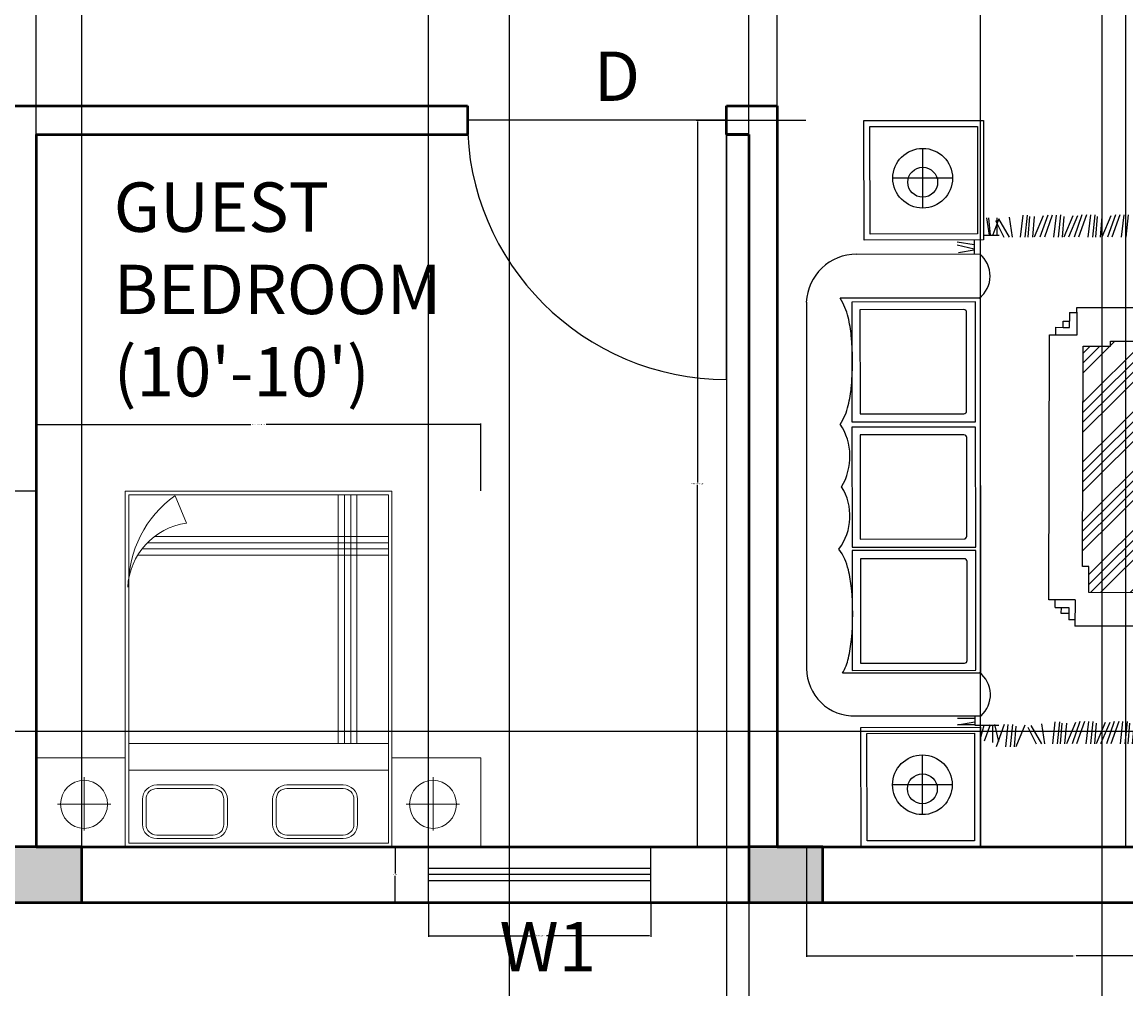
# Model space of a CAD drawing. Units: inches. Extents: x -1517 to -668, y -425 to 52.
# Tile 3 of 13: x -1365 to -1186, y -296 to -140. Entities that reach past the tile are written whole.
import ezdxf

# ---------------------------------------------------------------- set-up
doc = ezdxf.new("R2010")
doc.units = ezdxf.units.IN
doc.header["$MEASUREMENT"] = 0
for name, color, linetype, lineweight in [('A-ANNO-DIMS', 2, 'Continuous', 18), ('A-ANNO-TEXT', 7, 'Continuous', 18), ('A-AREA-IDEN', 7, 'Continuous', 25), ('A-COLS-PATT', 252, 'Continuous', 13), ('column', 7, 'Continuous', 50), ('doors', 25, 'Continuous', 25), ('furniture block', 8, 'Continuous', 18), ('walls', 240, 'Continuous', 50), ('windows', 140, 'Continuous', 25)]:
    doc.layers.add(name, color=color, linetype=linetype, lineweight=lineweight)
for name, color, linetype in [('复线', 6, 'Continuous'), ('家具', 4, 'Continuous'), ('辅助线', 1, 'Continuous'), ('门窗', 2, 'Continuous')]:
    doc.layers.add(name, color=color, linetype=linetype)
doc.styles.get("Standard").update_dxf_attribs({"font": 'arial.ttf'})
doc.dimstyles.get("Standard").update_dxf_attribs({"dimtxt": 0.18, "dimasz": 0.18, "dimexe": 0.18, "dimexo": 0.0625, "dimgap": 0.09, "dimtad": 0, "dimtih": 1, "dimtoh": 1, "dimdec": 4, "dimzin": 0, "dimdsep": 46, "dimlunit": 4, "dimtxsty": 'Standard', "dimcen": 0.09, "dimadec": 0, "dimazin": 0, "dimtfac": 1, "dimtdec": 4, "dimtofl": 0, "dimtmove": 0, "dimatfit": 3, "dimfxl": 1, "dimtolj": 1, "dimtzin": 0, "dimarcsym": 0})

# ---------------------------------------------------------------- blocks, each defined once
blk = doc.blocks.new('door 3.6ft')
for p, q in [((0, 42), (0, 0)), ((0, 0), (42, 0))]:
    blk.add_line(p, q)
blk.add_arc((0, 0), 42, 0, 90)
blk = doc.blocks.new('column')
for p, q in [((0, 9), (0, 0)), ((12, 9), (0, 9)), ((12, 0), (12, 9)), ((0, 0), (12, 0))]:
    blk.add_line(p, q)
blk = doc.blocks.new('window 3ft')
for p, q in [((9, 36), (0, 36)), ((3.5, 36), (3.5, 0)), ((4.5, 36), (4.5, 0)), ((5.5, 36), (5.5, 0)), ((9, 0), (0, 0))]:
    blk.add_line(p, q)
blk = doc.blocks.new('A$C057D194F')
for p, q in [((0, 1.5, -0.1688), (0, 2, -0.1688)), ((0, 2, -0.1688), (0.5, 2, -0.1688)), ((0.5, 2, -0.1688), (0.5, 0, -0.1688)), ((2, 2, -0.1688), (0.5, 2, -0.1688)), ((2, 0, -0.1688), (2, 2, -0.1688)), ((2.5, 2, -0.1688), (2, 2, -0.1688)), ((2.5, 1.5, -0.1688), (2.5, 2, -0.1688)), ((1.98, 1.98, -0.1688), (0.52, 1.98, -0.1688)), ((0.52, 1.98, -0.1688), (0.52, 0.02, -0.1688)), ((1.0907, 1.9539, -0.1688), (0.7735, 1.9539, -0.1688)), ((1.0907, 1.9339, -0.1688), (0.7735, 1.9339, -0.1688)), ((1.8224, 1.9539, -0.1688), (1.5052, 1.9539, -0.1688)), ((1.8224, 1.9339, -0.1688), (1.5052, 1.9339, -0.1688)), ((1.98, 0.02, -0.1688), (1.98, 1.98, -0.1688)), ((0.2687, 1.9081, -0.1688), (0.2687, 1.761, -0.1688)), ((0.2687, 1.6081, -0.1688), (0.2687, 1.9081, -0.1688)), ((0.6935, 1.8739, -0.1688), (0.6935, 1.7322, -0.1688)), ((0.7135, 1.8739, -0.1688), (0.7135, 1.7322, -0.1688)), ((1.1507, 1.7322, -0.1688), (1.1507, 1.8739, -0.1688)), ((1.1707, 1.7322, -0.1688), (1.1707, 1.8739, -0.1688)), ((1.4252, 1.8739, -0.1688), (1.4252, 1.7322, -0.1688)), ((1.4452, 1.8739, -0.1688), (1.4452, 1.7322, -0.1688)), ((1.8824, 1.7322, -0.1688), (1.8824, 1.8739, -0.1688)), ((1.9024, 1.7322, -0.1688), (1.9024, 1.8739, -0.1688)), ((2.2313, 1.9081, -0.1688), (2.2313, 1.761, -0.1688)), ((2.2313, 1.6081, -0.1688), (2.2313, 1.9081, -0.1688)), ((0.4194, 1.761, -0.1688), (0.1194, 1.761, -0.1688)), ((0.2687, 1.761, -0.1688), (0.4194, 1.761, -0.1688)), ((0.2687, 1.761, -0.1688), (0.2687, 1.6081, -0.1688)), ((2.0806, 1.761, -0.1688), (2.3806, 1.761, -0.1688)), ((2.2313, 1.761, -0.1688), (2.0806, 1.761, -0.1688)), ((2.2313, 1.761, -0.1688), (2.2313, 1.6081, -0.1688)), ((0.7735, 1.6722, -0.1688), (1.0907, 1.6722, -0.1688)), ((0.7735, 1.6522, -0.1688), (1.0907, 1.6522, -0.1688)), ((1.5052, 1.6722, -0.1688), (1.8224, 1.6722, -0.1688)), ((1.5052, 1.6522, -0.1688), (1.8224, 1.6522, -0.1688)), ((1.98, 1.5693, -0.1688), (0.52, 1.5693, -0.1688)), ((0.5, 1.5, -0.1688), (0, 1.5, -0.1688)), ((2, 1.5, -0.1688), (2.5, 1.5, -0.1688)), ((1.98, 1.4193, -0.1688), (0.52, 1.4193, -0.1688)), ((0.6969, 0.02, -0.1688), (0.6969, 1.4193, -0.1688)), ((0.7319, 0.02, -0.1688), (0.7319, 1.4193, -0.1688)), ((0.7669, 0.02, -0.1688), (0.7669, 1.4193, -0.1688)), ((0.8019, 0.02, -0.1688), (0.8019, 1.4193, -0.1688)), ((0.52, 0.3595, -0.1688), (1.9292, 0.3595, -0.1688)), ((0.52, 0.3245, -0.1688), (1.905, 0.3245, -0.1688)), ((0.52, 0.2895, -0.1688), (1.8742, 0.2895, -0.1688)), ((0.52, 0.2545, -0.1688), (1.8344, 0.2545, -0.1688)), ((1.6548, 0.1789, -0.1688), (1.7198, 0.0251, -0.1688)), ((0.52, 0.02, -0.1688), (1.98, 0.02, -0.1688)), ((0.5, 0, -0.1688), (2, 0, -0.1688))]:
    blk.add_line(p, q)
for centre, radius, start, end in [((0.7735, 1.8739, -0.1688), 0.08, 90, 180), ((0.7735, 1.8739, -0.1688), 0.06, 90, 180), ((1.0907, 1.8739, -0.1688), 0.08, 0, 90), ((1.0907, 1.8739, -0.1688), 0.06, 0, 90), ((1.5052, 1.8739, -0.1688), 0.08, 90, 180), ((1.5052, 1.8739, -0.1688), 0.06, 90, 180), ((1.8224, 1.8739, -0.1688), 0.08, 0, 90), ((1.8224, 1.8739, -0.1688), 0.06, 0, 90), ((0.7735, 1.7322, -0.1688), 0.08, 180, 270), ((0.7735, 1.7322, -0.1688), 0.06, 180, 270), ((1.0907, 1.7322, -0.1688), 0.08, 270, 0), ((1.0907, 1.7322, -0.1688), 0.06, 270, 0), ((1.5052, 1.7322, -0.1688), 0.08, 180, 270), ((1.5052, 1.7322, -0.1688), 0.06, 180, 270), ((1.8224, 1.7322, -0.1688), 0.08, 270, 0), ((1.8224, 1.7322, -0.1688), 0.06, 270, 0), ((1.5992, 0.5623, -0.1688), 0.3874, 278.2518, 356.6808), ((1.363, 0.5286, -0.1688), 0.6171, 305.32946, 1.04595)]:
    blk.add_arc(centre, radius, start, end)
blk.add_ellipse((0.2687, 1.761, -0.1688), major_axis=(0, -0.1351), ratio=0.975448)
at = {"extrusion": (0, 0, -1)}
blk.add_ellipse((2.2313, 1.761, -0.1688), major_axis=(0, 0.1351), ratio=0.975448, dxfattribs=at)
for p in [(0.2687, 1.761, -0.1688), (2.2313, 1.761, -0.1688)]:
    blk.add_point(p)
blk = doc.blocks.new('A$C2A9E403C')
at = {"layer": '复线'}
for p, q in [((-0.4956, 1.5596), (0.4554, 1.5575)), ((-0.4956, 1.5385), (-0.4956, 1.5596)), ((0.4554, 1.5575), (0.4547, 1.198)), ((-0.6124, 1.2901), (-0.6119, 1.5387)), ((-0.6119, 1.5387), (-0.4956, 1.5385)), ((-0.5913, 1.2901), (-0.6124, 1.2901)), ((-0.5915, 1.1738), (-0.5913, 1.2901)), ((0.3437, 1.1718), (-0.5915, 1.1738)), ((0.3437, 1.1982), (0.3437, 1.1718)), ((0.4547, 1.198), (0.3437, 1.1982)), ((0.7969, 0.7406), (-0.7994, 0.7387)), ((-0.27, 0.7177), (-0.7787, 0.7173)), ((-0.7787, 0.7173), (-0.7783, 0.1924)), ((-0.2696, 0.1928), (-0.27, 0.7177)), ((0.2616, 0.7183), (-0.2471, 0.718)), ((-0.2471, 0.718), (-0.2468, 0.1931)), ((0.2619, 0.1934), (0.2616, 0.7183)), ((0.7846, 0.7189), (0.2759, 0.7186)), ((0.2759, 0.7186), (0.2762, 0.1937)), ((0.785, 0.194), (0.7846, 0.7189)), ((-1.3039, 0.62), (-1.3039, 0.3666)), ((1.2704, 0.6186), (1.2704, 0.3652)), ((-1.1772, 0.4933), (-1.4306, 0.4933)), ((1.3971, 0.4919), (1.1437, 0.4919)), ((-0.7783, 0.1924), (-0.2696, 0.1928)), ((-0.2468, 0.1931), (0.2619, 0.1934)), ((0.2762, 0.1937), (0.785, 0.194))]:
    blk.add_line(p, q, dxfattribs=at)
for centre in [(-1.2867, 0.4933), (1.2877, 0.4919)]:
    blk.add_circle(centre, 0.0634, dxfattribs=at)
at = {"layer": '家具'}
for p, q in [((0.6497, 2.19), (0.6526, 2.1827)), ((-0.6379, 1.6813), (-0.6378, 1.7025)), ((-0.6378, 1.7025), (0.4874, 1.7)), ((0.4874, 1.7), (0.4872, 1.5943)), ((-0.6961, 1.655), (-0.6696, 1.655)), ((-0.6961, 1.6233), (-0.6961, 1.655)), ((-0.6696, 1.6814), (-0.6379, 1.6813)), ((-0.6696, 1.655), (-0.6696, 1.6814)), ((-0.6694, 1.655), (-0.6694, 1.6235)), ((-0.6378, 1.6814), (-0.6379, 1.597)), ((0.519, 1.6788), (0.4873, 1.6789)), ((0.5189, 1.6154), (0.519, 1.6788)), ((0.519, 1.6524), (0.5507, 1.6523)), ((0.5507, 1.6523), (0.5506, 1.6153)), ((-0.7553, 1.1479), (-0.7543, 1.597)), ((-0.7543, 1.597), (-0.7279, 1.597)), ((-0.6379, 1.597), (-0.7282, 1.5972)), ((-0.7279, 1.597), (-0.7278, 1.6234)), ((-0.7278, 1.6234), (-0.6961, 1.6233)), ((-0.6694, 1.6235), (-0.6966, 1.6235)), ((0.4872, 1.5943), (0.5981, 1.5941)), ((0.5717, 1.6153), (0.5189, 1.6154)), ((0.5717, 1.6153), (0.5717, 1.5941)), ((0.5981, 1.5941), (0.5971, 1.1396)), ((-0.7341, 1.1478), (-0.7553, 1.1479)), ((-0.6393, 1.1482), (-0.7352, 1.1484)), ((-0.7342, 1.1161), (-0.7341, 1.1478)), ((-0.6394, 1.058), (-0.6393, 1.1482)), ((0.4862, 1.1399), (0.4859, 1.0289)), ((0.4862, 1.1399), (0.5971, 1.1396)), ((0.5707, 1.1397), (0.5706, 1.1133)), ((-0.7342, 1.1161), (-0.6972, 1.116)), ((-0.6709, 1.116), (-0.6979, 1.1161)), ((-0.6973, 1.0896), (-0.6972, 1.116)), ((-0.6709, 1.0896), (-0.6973, 1.0896)), ((-0.671, 1.0579), (-0.6709, 1.0896)), ((-0.6709, 1.0896), (-0.6709, 1.116)), ((0.5177, 1.0553), (0.5178, 1.1134)), ((0.5441, 1.0816), (0.5177, 1.0817)), ((0.5178, 1.1134), (0.5706, 1.1133)), ((0.5442, 1.1133), (0.5441, 1.0816)), ((-0.6393, 1.0578), (-0.671, 1.0579)), ((-0.6393, 1.0314), (-0.6393, 1.0578)), ((0.4859, 1.0289), (-0.6393, 1.0314)), ((0.5177, 1.0553), (0.486, 1.0553)), ((-1.549, 0.751), (-1.0422, 0.7516)), ((-1.5485, 0.2441), (-1.549, 0.751)), ((-1.0422, 0.7516), (-1.0416, 0.2447)), ((-0.9818, 0.2137), (-0.9824, 0.7352)), ((-0.7945, 0.7328), (-0.7941, 0.1426)), ((0.7969, 0.7406), (0.7973, 0.1532)), ((0.9782, 0.2083), (0.9775, 0.741)), ((1.0263, 0.7379), (1.5332, 0.7385)), ((1.0269, 0.2311), (1.0263, 0.7379)), ((1.5332, 0.7385), (1.5338, 0.2316)), ((-1.0416, 0.2447), (-1.5485, 0.2441)), ((1.5338, 0.2316), (1.0269, 0.2311)), ((-0.7773, -0.0005), (0.7773, 0.0005))]:
    blk.add_line(p, q, dxfattribs=at)
for centre in [(-1.3039, 0.4933), (1.2704, 0.4919)]:
    blk.add_circle(centre, 0.1267, dxfattribs=at)
for centre, radius, start, end in [((-0.8894, 0.6597), 0.1198, 37.63, 140.9463), ((0.8885, 0.6609), 0.1198, 41.7931, 142.4463), ((-0.7672, 0.2138), 0.2146, 180.0381, 267.3174), ((0.7771, 0.2016), 0.2011, 270.0381, 1.8876), ((-0.6554, -0.0689), 0.253, 103.3408, 123.2571), ((-0.3975, -0.0687), 0.253, 56.8202, 76.7354), ((-0.1227, -0.0686), 0.253, 59.3987, 122.9427), ((0.1299, -0.0495), 0.2341, 53.2114, 121.9243), ((0.4167, -0.0682), 0.253, 103.3408, 125.4146), ((0.6746, -0.068), 0.253, 60.9819, 76.7354)]:
    blk.add_arc(centre, radius, start, end, dxfattribs=at)
at = {"layer": '辅助线'}
for p, q in [((-1.0661, 2.2523), (-1.0302, 2.1808)), ((-1.0533, 2.2588), (-1.0079, 2.1808)), ((-1.0082, 2.2653), (-0.9957, 2.1808)), ((-0.9309, 2.2654), (-0.9778, 2.1808)), ((-0.8827, 2.2686), (-0.8899, 2.1809)), ((-0.8633, 2.2687), (-0.8705, 2.181)), ((-0.8247, 2.2719), (-0.8633, 2.181)), ((-0.8054, 2.2752), (-0.8391, 2.181)), ((-0.7861, 2.2752), (-0.8197, 2.181)), ((-0.77, 2.2752), (-0.7803, 2.1811)), ((-0.7507, 2.2752), (-0.761, 2.1811)), ((-0.741, 2.2688), (-0.7482, 2.1811)), ((-0.7217, 2.2688), (-0.7289, 2.1811)), ((-0.6831, 2.2721), (-0.7216, 2.1811)), ((-0.6638, 2.2753), (-0.6974, 2.1812)), ((-0.6444, 2.2753), (-0.6781, 2.1812)), ((-0.6284, 2.2754), (-0.6387, 2.1812)), ((-0.609, 2.2754), (-0.6194, 2.1812)), ((-0.5189, 2.253), (-0.483, 2.1814)), ((-0.506, 2.2594), (-0.4607, 2.1814)), ((-0.4609, 2.2659), (-0.4484, 2.1814)), ((-0.4036, 2.2756), (-0.414, 2.1815)), ((-0.3843, 2.2757), (-0.3946, 2.1815)), ((-0.3746, 2.2692), (-0.3818, 2.1815)), ((-0.3553, 2.2693), (-0.3625, 2.1815)), ((-0.3167, 2.2725), (-0.3552, 2.1816)), ((-0.2974, 2.2758), (-0.331, 2.1816)), ((-0.278, 2.2758), (-0.3117, 2.1816)), ((-0.262, 2.2758), (-0.2723, 2.1816)), ((-0.2426, 2.2758), (-0.253, 2.1817)), ((-0.2292, 2.2694), (-0.2364, 2.1817)), ((-0.1906, 2.2727), (-0.2291, 2.1817)), ((-0.1712, 2.2727), (-0.2098, 2.1817)), ((-0.1519, 2.2759), (-0.1856, 2.1817)), ((-0.1326, 2.2759), (-0.1663, 2.1818)), ((-0.1165, 2.276), (-0.1269, 2.1818)), ((-0.0972, 2.276), (-0.1076, 2.1818)), ((-0.0875, 2.2696), (-0.0948, 2.1819)), ((-0.0682, 2.2696), (-0.0754, 2.1819)), ((-0.0296, 2.2728), (-0.0682, 2.1819)), ((-0.0103, 2.2761), (-0.044, 2.1819)), ((0.009, 2.2761), (-0.0246, 2.1819)), ((0.0251, 2.2761), (0.0148, 2.182)), ((0.0444, 2.2761), (0.0341, 2.182)), ((0.1539, 2.2634), (0.154, 2.1821)), ((0.17, 2.2634), (0.1701, 2.1822)), ((0.199, 2.2635), (0.1882, 2.1822)), ((0.2279, 2.2635), (0.228, 2.1822)), ((0.244, 2.2635), (0.2441, 2.1822)), ((0.273, 2.2635), (0.2623, 2.1823)), ((0.2891, 2.2636), (0.2783, 2.1823)), ((0.2923, 2.2636), (0.3127, 2.1823)), ((0.3084, 2.2636), (0.3288, 2.1823)), ((0.3148, 2.2668), (0.3657, 2.1824)), ((0.3309, 2.2668), (0.3818, 2.1824)), ((0.4018, 2.2701), (0.3945, 2.1824)), ((0.4211, 2.2702), (0.4139, 2.1824)), ((0.4597, 2.2734), (0.4211, 2.1825)), ((0.479, 2.2767), (0.4453, 2.1825)), ((0.4983, 2.2767), (0.4647, 2.1825)), ((0.5144, 2.2767), (0.5041, 2.1825)), ((0.5337, 2.2767), (0.5234, 2.1826)), ((0.6175, 2.2543), (0.6497, 2.19)), ((0.6303, 2.2607), (0.6756, 2.1827)), ((0.6754, 2.2672), (0.6879, 2.1828)), ((0.7526, 2.2673), (0.7058, 2.1828)), ((0.7668, 2.187), (0.7667, 2.2602)), ((0.8009, 2.2642), (0.801, 2.1829)), ((0.846, 2.2642), (0.8352, 2.1829)), ((0.8653, 2.2642), (0.8857, 2.183)), ((0.8878, 2.2675), (0.9387, 2.1831)), ((0.92, 2.2643), (0.9405, 2.1831)), ((0.9426, 2.2675), (0.9934, 2.1831)), ((-1.1526, 2.1822), (-1.0649, 2.175)), ((1.1031, 2.1597), (1.0154, 2.1669)), ((-1.1494, 2.1339), (-1.0648, 2.0871)), ((1.1031, 2.1404), (1.0154, 2.1476)), ((1.1064, 2.1018), (1.0154, 2.1404)), ((1.1096, 2.0825), (1.0155, 2.1161)), ((-1.1493, 2.0567), (-1.0648, 2.0692)), ((1.1097, 2.0632), (1.0155, 2.0968)), ((-1.1428, 2.0116), (-1.0648, 2.0569)), ((-1.1205, 2.0067), (-1.0648, 2.0347)), ((1.1097, 2.0471), (1.0155, 2.0574)), ((1.1097, 2.0278), (1.0156, 2.0381)), ((-1.1354, 1.9942), (-1.0477, 1.987)), ((-1.1354, 1.9749), (-1.0477, 1.9677)), ((1.0017, 1.9919), (1.0958, 1.9816)), ((1.0017, 1.9726), (1.0958, 1.9623)), ((-1.1321, 1.9041), (-1.0476, 1.9549)), ((-1.132, 1.888), (-1.0476, 1.9389)), ((1.0017, 1.9565), (1.0959, 1.9229)), ((1.0017, 1.9372), (1.0959, 1.9036)), ((-1.1288, 1.8816), (-1.0476, 1.902)), ((-1.1288, 1.8655), (-1.0476, 1.8859)), ((1.005, 1.9179), (1.0959, 1.8793)), ((1.0082, 1.8793), (1.0959, 1.8721)), ((-1.1487, 1.855), (-1.0545, 1.8446)), ((-1.1486, 1.8356), (-1.0545, 1.8253)), ((-1.1288, 1.8623), (-1.0475, 1.8515)), ((-1.1288, 1.8462), (-1.0475, 1.8354)), ((1.0083, 1.86), (1.096, 1.8528)), ((1.0116, 1.7892), (1.096, 1.84)), ((-1.1486, 1.8196), (-1.0544, 1.7859)), ((-1.1486, 1.8002), (-1.0544, 1.7666)), ((-1.1454, 1.7809), (-1.0544, 1.7424)), ((-1.1287, 1.8172), (-1.0475, 1.8173)), ((-1.1287, 1.8011), (-1.0475, 1.8012)), ((1.0116, 1.7731), (1.096, 1.8239)), ((1.0148, 1.7666), (1.096, 1.787)), ((-1.1421, 1.7423), (-1.0544, 1.7351)), ((-1.1287, 1.7721), (-1.0474, 1.7614)), ((-1.1287, 1.7432), (-1.0474, 1.7433)), ((1.0148, 1.7505), (1.0961, 1.771)), ((1.0148, 1.7473), (1.0961, 1.7366)), ((-1.1421, 1.723), (-1.0544, 1.7158)), ((-1.1388, 1.6522), (-1.0544, 1.703)), ((-1.1388, 1.6361), (-1.0543, 1.6869)), ((-1.1286, 1.7271), (-1.0474, 1.7272)), ((1.0148, 1.7312), (1.0961, 1.7205)), ((1.0149, 1.7022), (1.0961, 1.7023)), ((-1.1355, 1.6296), (-1.0543, 1.6501)), ((1.0149, 1.6861), (1.0962, 1.6862)), ((1.0149, 1.6572), (1.0962, 1.6464)), ((-1.1355, 1.6135), (-1.0543, 1.634)), ((-1.1355, 1.6103), (-1.0542, 1.5996)), ((-1.1355, 1.5942), (-1.0542, 1.5835)), ((1.015, 1.6282), (1.0962, 1.6283)), ((1.015, 1.6121), (1.0962, 1.6122)), ((-1.1355, 1.5653), (-1.0542, 1.5654)), ((-1.1354, 1.5492), (-1.0542, 1.5493)), ((-0.0998, 1.1727), (-0.4849, 1.5596)), ((-0.0578, 1.1727), (-0.4429, 1.5595)), ((-0.0158, 1.1726), (-0.4009, 1.5594)), ((0.0262, 1.1725), (-0.3589, 1.5593)), ((0.1522, 1.1722), (-0.2329, 1.559)), ((0.1942, 1.1721), (-0.1909, 1.5589)), ((0.2362, 1.172), (-0.1489, 1.5588)), ((0.2782, 1.1719), (-0.1069, 1.5587)), ((0.3779, 1.1981), (0.0191, 1.5585)), ((0.4199, 1.198), (0.0611, 1.5584)), ((0.4547, 1.2052), (0.1031, 1.5583)), ((0.4548, 1.2472), (0.1451, 1.5582)), ((0.455, 1.3732), (0.2711, 1.5579)), ((0.4551, 1.4152), (0.3131, 1.5578)), ((0.4552, 1.4572), (0.3551, 1.5577)), ((0.4553, 1.4992), (0.3971, 1.5576)), ((-1.1354, 1.5202), (-1.0541, 1.5094)), ((-0.2678, 1.1731), (-0.6119, 1.5187)), ((-0.2258, 1.173), (-0.5898, 1.5387)), ((1.0022, 1.5026), (1.0964, 1.4923)), ((-1.1354, 1.4912), (-1.0541, 1.4913)), ((-1.1354, 1.4751), (-1.0541, 1.4752)), ((-0.3098, 1.1732), (-0.612, 1.4767)), ((1.0023, 1.4833), (1.0964, 1.473)), ((1.0023, 1.4672), (1.0965, 1.4336)), ((-0.3518, 1.1733), (-0.6121, 1.4347)), ((1.0023, 1.4479), (1.0965, 1.4143)), ((1.0055, 1.4286), (1.0965, 1.39)), ((-1.1481, 1.3657), (-1.0539, 1.3553)), ((1.0024, 1.361), (1.0966, 1.3506)), ((1.0088, 1.39), (1.0965, 1.3828)), ((1.0088, 1.3707), (1.0965, 1.3635)), ((-1.1481, 1.3463), (-1.0539, 1.336)), ((-1.1481, 1.3303), (-1.0539, 1.2966)), ((1.0024, 1.3417), (1.0966, 1.3313)), ((1.0024, 1.3256), (1.0966, 1.2919)), ((-1.148, 1.3109), (-1.0539, 1.2773)), ((-1.1448, 1.2916), (-1.0538, 1.2531)), ((-0.5938, 1.2901), (-0.6124, 1.3087)), ((-0.4778, 1.1736), (-0.5913, 1.2876)), ((1.0025, 1.3063), (1.0966, 1.2726)), ((1.0057, 1.287), (1.0967, 1.2484)), ((1.0057, 1.2677), (1.0967, 1.2291)), ((-1.1479, 1.224), (-1.0538, 1.2137)), ((-1.1415, 1.253), (-1.0538, 1.2458)), ((-1.1415, 1.2337), (-1.0538, 1.2265)), ((-0.5198, 1.1737), (-0.5914, 1.2456)), ((1.009, 1.229), (1.0967, 1.2218)), ((-1.1479, 1.2047), (-1.0538, 1.1944)), ((-1.1479, 1.1886), (-1.0537, 1.155)), ((-0.5618, 1.1738), (-0.5915, 1.2036)), ((1.0026, 1.2156), (1.0967, 1.2052)), ((1.0026, 1.1963), (1.0967, 1.1859)), ((1.0026, 1.1802), (1.0968, 1.1465)), ((-1.1479, 1.1693), (-1.0537, 1.1356)), ((-1.1446, 1.15), (-1.0537, 1.1114)), ((-1.1446, 1.1307), (-1.0536, 1.0921)), ((1.0026, 1.1608), (1.0968, 1.1272)), ((1.0059, 1.1415), (1.0968, 1.103)), ((-1.1478, 1.0786), (-1.0536, 1.0682)), ((-1.1413, 1.0921), (-1.0536, 1.0848)), ((1.0091, 1.1029), (1.0968, 1.0957)), ((1.0092, 1.0836), (1.0969, 1.0764)), ((-1.1477, 1.0593), (-1.0536, 1.0489)), ((-1.1477, 1.0432), (-1.0535, 1.0095)), ((1.0027, 1.0739), (1.0969, 1.0636)), ((1.0028, 1.0546), (1.0969, 1.0443)), ((-1.1477, 1.0239), (-1.0535, 0.9902)), ((-1.1445, 1.0046), (-1.0535, 0.966)), ((1.0125, 0.9973), (1.0969, 1.0098)), ((1.019, 0.9522), (1.097, 0.9975)), ((-1.1476, 0.937), (-1.0535, 0.9266)), ((-1.1412, 0.9659), (-1.0535, 0.9587)), ((-1.1412, 0.9466), (-1.0535, 0.9394)), ((1.0254, 0.9393), (1.097, 0.9752)), ((-1.1476, 0.9176), (-1.0534, 0.9073)), ((1.0182, 0.9266), (1.1091, 0.8881)), ((-1.1379, 0.8603), (-1.0534, 0.8728)), ((-1.1314, 0.8152), (-1.0534, 0.8605)), ((1.015, 0.8745), (1.1091, 0.8642)), ((1.015, 0.8552), (1.1092, 0.8449)), ((1.0214, 0.888), (1.1091, 0.8808)), ((-1.1353, 0.8078), (-1.062, 0.8079)), ((-1.132, 0.8163), (-1.0631, 0.7916)), ((-1.1249, 0.8024), (-1.0533, 0.8383)), ((-1.0607, 0.8176), (-1.0606, 0.7516)), ((1.015, 0.8391), (1.1092, 0.8055)), ((1.0151, 0.7984), (1.0863, 0.8153)), ((1.0173, 0.7141), (1.0171, 0.8166)), ((-1.1351, 0.7732), (-1.0621, 0.7791)), ((-1.135, 0.7635), (-1.0628, 0.7759)), ((1.0164, 0.7803), (1.0847, 0.754)), ((1.0174, 0.7888), (1.0906, 0.7889)), ((1.0189, 0.7534), (1.0705, 0.738)), ((-1.5237, 0.7257), (-1.0675, 0.7262)), ((-1.5231, 0.2695), (-1.5237, 0.7257)), ((-1.0675, 0.7262), (-1.067, 0.27)), ((-1.0421, 0.7117), (-0.9824, 0.7118)), ((-1.0339, 0.6392), (-1.0219, 0.7114)), ((-1.0207, 0.6402), (-1.0046, 0.7117)), ((-0.9891, 0.6447), (-1.0003, 0.7117)), ((0.9776, 0.714), (1.0173, 0.7141)), ((0.988, 0.6409), (0.9879, 0.7142)), ((1.0156, 0.6423), (1.004, 0.7146)), ((1.0149, 0.641), (1.0148, 0.7142)), ((1.0517, 0.7126), (1.5079, 0.7131)), ((1.0522, 0.2564), (1.0517, 0.7126)), ((1.5079, 0.7131), (1.5084, 0.257)), ((-0.7461, 0.6679), (-0.7458, 0.227)), ((-0.316, 0.6798), (-0.7345, 0.6795)), ((-0.3041, 0.2273), (-0.3044, 0.6682)), ((-0.2146, 0.6685), (-0.2143, 0.2277)), ((0.2155, 0.6804), (-0.203, 0.6801)), ((0.2275, 0.228), (0.2272, 0.6688)), ((0.3111, 0.6701), (0.3114, 0.2287)), ((0.7428, 0.682), (0.3227, 0.6817)), ((0.7547, 0.229), (0.7544, 0.6704)), ((-1.067, 0.27), (-1.5231, 0.2695)), ((1.5084, 0.257), (1.0522, 0.2564)), ((-0.7458, 0.227), (-0.3041, 0.2273)), ((-0.2143, 0.2277), (0.2275, 0.228)), ((0.3114, 0.2287), (0.7547, 0.229))]:
    blk.add_line(p, q, dxfattribs=at)
for centre, start, end in [((-0.7345, 0.6679), 90.0381, 180.0381), ((-0.316, 0.6682), 0.0381, 90.0381), ((-0.203, 0.6685), 90.0381, 180.0381), ((0.2156, 0.6688), 0.0381, 90.0381), ((0.3228, 0.6701), 90.0381, 180.0381), ((0.7428, 0.6703), 0.0381, 90.0381)]:
    blk.add_arc(centre, 0.0116, start, end, dxfattribs=at)
at = {"layer": '门窗'}
for centre, radius, start, end in [((-0.5778, -0.396), 0.5891, 95.6316, 103.3408), ((-0.5259, -0.9226), 1.1183, 84.4446, 95.6316), ((-0.4747, -0.3959), 0.5891, 76.7354, 84.4446), ((0.4943, -0.3953), 0.5891, 95.6316, 103.3408), ((0.5462, -0.9219), 1.1183, 84.4446, 95.6316), ((0.5974, -0.3952), 0.5891, 76.7354, 84.4446)]:
    blk.add_arc(centre, radius, start, end, dxfattribs=at)
blk = doc.blocks.new('*D18')
at = {"layer": 'A-ANNO-DIMS', "color": 0, "lineweight": -2, "transparency": 16777216}
for p, q in [((-1298.98, -282.43), (-1298.98, -287.95)), ((-1262.98, -282.43), (-1262.98, -287.95)), ((-1298.8, -287.77), (-1282.1, -287.77)), ((-1263.16, -287.77), (-1279.86, -287.77))]:
    blk.add_line(p, q, dxfattribs=at)
at = {"layer": 'A-ANNO-DIMS', "color": 0, "transparency": 16777216}
for points in [[(-1298.8, -287.74), (-1298.8, -287.8), (-1298.98, -287.77)], [(-1263.16, -287.74), (-1263.16, -287.8), (-1262.98, -287.77)]]:
    blk.add_solid(points, dxfattribs=at)
at = {"layer": 'Defpoints', "color": 0, "transparency": 16777216}
for p in [(-1298.98, -282.37), (-1262.98, -282.37), (-1262.98, -287.77)]:
    blk.add_point(p, dxfattribs=at)
at = {"layer": 'A-ANNO-DIMS', "color": 0, "transparency": 16777216, "insert": (-1280.98, -287.77), "char_height": 0.18, "attachment_point": 5}
blk.add_mtext('\\A1;WINDOW 36 TYP.', dxfattribs=at)
blk = doc.blocks.new('*D19')
at = {"layer": 'A-ANNO-DIMS', "color": 0, "lineweight": -2, "transparency": 16777216}
for p, q in [((-1299.04, -273.37), (-1304.56, -273.37)), ((-1304.38, -273.55), (-1304.38, -277.69)), ((-1304.38, -282.19), (-1304.38, -278.05)), ((-1299.04, -282.37), (-1304.56, -282.37))]:
    blk.add_line(p, q, dxfattribs=at)
at = {"layer": 'A-ANNO-DIMS', "color": 0, "transparency": 16777216}
for points in [[(-1304.41, -273.55), (-1304.35, -273.55), (-1304.38, -273.37)], [(-1304.41, -282.19), (-1304.35, -282.19), (-1304.38, -282.37)]]:
    blk.add_solid(points, dxfattribs=at)
at = {"layer": 'Defpoints', "color": 0, "transparency": 16777216}
for p in [(-1298.98, -273.37), (-1304.38, -282.37), (-1298.98, -282.37)]:
    blk.add_point(p, dxfattribs=at)
at = {"layer": 'A-ANNO-DIMS', "color": 0, "transparency": 16777216, "insert": (-1304.38, -277.87), "char_height": 0.18, "attachment_point": 5}
blk.add_mtext('\\A1;9 TYP.', dxfattribs=at)
blk = doc.blocks.new('*D40')
at = {"layer": 'A-ANNO-DIMS', "color": 0, "lineweight": -2, "transparency": 16777216}
for p, q in [((-1362.5, -215.71), (-1362.5, -204.79)), ((-1362.32, -204.97), (-1327.76, -204.97)), ((-1290.68, -204.97), (-1325.25, -204.97)), ((-1290.5, -215.71), (-1290.5, -204.79))]:
    blk.add_line(p, q, dxfattribs=at)
at = {"layer": 'A-ANNO-DIMS', "color": 0, "transparency": 16777216}
for points in [[(-1362.32, -204.94), (-1362.32, -205), (-1362.5, -204.97)], [(-1290.68, -204.94), (-1290.68, -205), (-1290.5, -204.97)]]:
    blk.add_solid(points, dxfattribs=at)
at = {"layer": 'Defpoints', "color": 0, "transparency": 16777216}
for p in [(-1362.5, -204.97), (-1362.5, -215.77), (-1290.5, -215.77)]:
    blk.add_point(p, dxfattribs=at)
at = {"layer": 'A-ANNO-DIMS', "color": 0, "transparency": 16777216, "insert": (-1326.5, -204.97), "char_height": 0.18, "attachment_point": 5}
blk.add_mtext('\\A1;GUEST BED SET 72', dxfattribs=at)
blk = doc.blocks.new('*D41')
at = {"layer": 'A-ANNO-DIMS', "color": 0, "lineweight": -2, "transparency": 16777216}
for p, q in [((-1362.57, -215.77), (-1373.48, -215.77)), ((-1373.3, -215.95), (-1373.3, -244.39)), ((-1373.3, -273.19), (-1373.3, -244.75)), ((-1362.57, -273.37), (-1373.48, -273.37))]:
    blk.add_line(p, q, dxfattribs=at)
at = {"layer": 'A-ANNO-DIMS', "color": 0, "transparency": 16777216}
for points in [[(-1373.33, -215.95), (-1373.27, -215.95), (-1373.3, -215.77)], [(-1373.33, -273.19), (-1373.27, -273.19), (-1373.3, -273.37)]]:
    blk.add_solid(points, dxfattribs=at)
at = {"layer": 'Defpoints', "color": 0, "transparency": 16777216}
for p in [(-1362.5, -215.77), (-1373.3, -273.37), (-1362.5, -273.37)]:
    blk.add_point(p, dxfattribs=at)
at = {"layer": 'A-ANNO-DIMS', "color": 0, "transparency": 16777216, "insert": (-1373.3, -244.57), "char_height": 0.18, "attachment_point": 5}
blk.add_mtext('\\A1;58', dxfattribs=at)
blk = doc.blocks.new('*D42')
at = {"layer": 'A-ANNO-DIMS', "color": 0, "lineweight": -2, "transparency": 16777216}
for p, q in [((-1237.84, -155.71), (-1255.61, -155.71)), ((-1255.43, -155.89), (-1255.43, -214.36)), ((-1255.43, -273.19), (-1255.43, -214.72)), ((-1237.84, -273.37), (-1255.61, -273.37))]:
    blk.add_line(p, q, dxfattribs=at)
at = {"layer": 'A-ANNO-DIMS', "color": 0, "transparency": 16777216}
for points in [[(-1255.46, -155.89), (-1255.4, -155.89), (-1255.43, -155.71)], [(-1255.46, -273.19), (-1255.4, -273.19), (-1255.43, -273.37)]]:
    blk.add_solid(points, dxfattribs=at)
at = {"layer": 'Defpoints', "color": 0, "transparency": 16777216}
for p in [(-1237.78, -155.71), (-1255.43, -273.37), (-1237.78, -273.37)]:
    blk.add_point(p, dxfattribs=at)
at = {"layer": 'A-ANNO-DIMS', "color": 0, "transparency": 16777216, "insert": (-1255.43, -214.54), "char_height": 0.18, "attachment_point": 5}
blk.add_mtext('\\A1;SOFA GROUP 118', dxfattribs=at)
blk = doc.blocks.new('*D43')
at = {"layer": 'A-ANNO-DIMS', "color": 0, "lineweight": -2, "transparency": 16777216}
for p, q in [((-1237.78, -273.43), (-1237.78, -291.2)), ((-1150.87, -273.43), (-1150.87, -291.2)), ((-1237.6, -291.02), (-1194.54, -291.02)), ((-1151.05, -291.02), (-1194.1, -291.02))]:
    blk.add_line(p, q, dxfattribs=at)
at = {"layer": 'A-ANNO-DIMS', "color": 0, "transparency": 16777216}
for points in [[(-1237.6, -290.99), (-1237.6, -291.05), (-1237.78, -291.02)], [(-1151.05, -290.99), (-1151.05, -291.05), (-1150.87, -291.02)]]:
    blk.add_solid(points, dxfattribs=at)
at = {"layer": 'Defpoints', "color": 0, "transparency": 16777216}
for p in [(-1237.78, -273.37), (-1150.87, -273.37), (-1150.87, -291.02)]:
    blk.add_point(p, dxfattribs=at)
at = {"layer": 'A-ANNO-DIMS', "color": 0, "transparency": 16777216, "insert": (-1194.32, -291.02), "char_height": 0.18, "attachment_point": 5}
blk.add_mtext('\\A1;87', dxfattribs=at)
blk = doc.blocks.new('*D48')
at = {"layer": 'A-ANNO-DIMS', "color": 0, "lineweight": -2, "transparency": 16777216}
for p, q in [((-1285.9, -102.43), (-1285.9, -376.85)), ((-1189.9, -102.43), (-1189.9, -376.85)), ((-1285.72, -376.67), (-1238.12, -376.67)), ((-1190.08, -376.67), (-1237.68, -376.67))]:
    blk.add_line(p, q, dxfattribs=at)
at = {"layer": 'A-ANNO-DIMS', "color": 0, "transparency": 16777216}
for points in [[(-1285.72, -376.64), (-1285.72, -376.7), (-1285.9, -376.67)], [(-1190.08, -376.64), (-1190.08, -376.7), (-1189.9, -376.67)]]:
    blk.add_solid(points, dxfattribs=at)
at = {"layer": 'Defpoints', "color": 0, "transparency": 16777216}
for p in [(-1285.9, -102.37), (-1189.9, -102.37), (-1189.9, -376.67)]:
    blk.add_point(p, dxfattribs=at)
at = {"layer": 'A-ANNO-DIMS', "color": 0, "transparency": 16777216, "insert": (-1237.9, -376.67), "char_height": 0.18, "attachment_point": 5}
blk.add_mtext('\\A1;96', dxfattribs=at)
blk = doc.blocks.new('*D52')
at = {"layer": 'A-ANNO-DIMS', "color": 0, "lineweight": -2, "transparency": 16777216}
for p, q in [((-1362.5, -157.91), (-1362.5, 52.11)), ((-1362.32, 51.93), (-1305.19, 51.93)), ((-1247.28, 51.93), (-1304.42, 51.93)), ((-1247.1, -157.91), (-1247.1, 52.11))]:
    blk.add_line(p, q, dxfattribs=at)
at = {"layer": 'A-ANNO-DIMS', "color": 0, "transparency": 16777216}
for points in [[(-1362.32, 51.96), (-1362.32, 51.9), (-1362.5, 51.93)], [(-1247.28, 51.96), (-1247.28, 51.9), (-1247.1, 51.93)]]:
    blk.add_solid(points, dxfattribs=at)
at = {"layer": 'Defpoints', "color": 0, "transparency": 16777216}
for p in [(-1247.1, 51.93), (-1362.5, -157.97), (-1247.1, -157.97)]:
    blk.add_point(p, dxfattribs=at)
at = {"layer": 'A-ANNO-DIMS', "color": 0, "transparency": 16777216, "insert": (-1304.8, 51.93), "char_height": 0.18, "attachment_point": 5}
blk.add_mtext('\\A1;115.4', dxfattribs=at)
blk = doc.blocks.new('*D53')
at = {"layer": 'A-ANNO-DIMS', "color": 0, "lineweight": -2, "transparency": 16777216}
for p, q in [((-1242.5, -153.31), (-1242.5, 52.11)), ((-1242.32, 51.93), (-1128.79, 51.93)), ((-1014.68, 51.93), (-1128.21, 51.93)), ((-1014.5, -150.31), (-1014.5, 52.11))]:
    blk.add_line(p, q, dxfattribs=at)
at = {"layer": 'A-ANNO-DIMS', "color": 0, "transparency": 16777216}
for points in [[(-1242.32, 51.96), (-1242.32, 51.9), (-1242.5, 51.93)], [(-1014.68, 51.96), (-1014.68, 51.9), (-1014.5, 51.93)]]:
    blk.add_solid(points, dxfattribs=at)
at = {"layer": 'Defpoints', "color": 0, "transparency": 16777216}
for p in [(-1014.5, 51.93), (-1014.5, -150.37), (-1242.5, -153.37)]:
    blk.add_point(p, dxfattribs=at)
at = {"layer": 'A-ANNO-DIMS', "color": 0, "transparency": 16777216, "insert": (-1128.5, 51.93), "char_height": 0.18, "attachment_point": 5}
blk.add_mtext('\\A1;228', dxfattribs=at)
blk = doc.blocks.new('*D64')
at = {"layer": 'A-ANNO-DIMS', "color": 0, "lineweight": -2, "transparency": 16777216}
for p, q in [((-1355.1, -282.31), (-1355.1, 52.11)), ((-1354.92, 51.93), (-1327.43, 51.93)), ((-1299.16, 51.93), (-1326.65, 51.93)), ((-1298.98, -282.31), (-1298.98, 52.11))]:
    blk.add_line(p, q, dxfattribs=at)
at = {"layer": 'A-ANNO-DIMS', "color": 0, "transparency": 16777216}
for points in [[(-1354.92, 51.96), (-1354.92, 51.9), (-1355.1, 51.93)], [(-1299.16, 51.96), (-1299.16, 51.9), (-1298.98, 51.93)]]:
    blk.add_solid(points, dxfattribs=at)
at = {"layer": 'Defpoints', "color": 0, "transparency": 16777216}
for p in [(-1298.98, 51.93), (-1355.1, -282.37), (-1298.98, -282.37)]:
    blk.add_point(p, dxfattribs=at)
at = {"layer": 'A-ANNO-DIMS', "color": 0, "transparency": 16777216, "insert": (-1327.04, 51.93), "char_height": 0.18, "attachment_point": 5}
blk.add_mtext('\\A1;56.12', dxfattribs=at)
blk = doc.blocks.new('*D66')
at = {"layer": 'A-ANNO-DIMS', "color": 0, "lineweight": -2, "transparency": 16777216}
for p, q in [((-1014.57, -254.68), (-1516.98, -254.68)), ((-1516.8, -254.86), (-1516.8, -263.85)), ((-1516.8, -273.19), (-1516.8, -264.21)), ((-1014.57, -273.37), (-1516.98, -273.37))]:
    blk.add_line(p, q, dxfattribs=at)
at = {"layer": 'A-ANNO-DIMS', "color": 0, "transparency": 16777216}
for points in [[(-1516.83, -254.86), (-1516.77, -254.86), (-1516.8, -254.68)], [(-1516.83, -273.19), (-1516.77, -273.19), (-1516.8, -273.37)]]:
    blk.add_solid(points, dxfattribs=at)
at = {"layer": 'Defpoints', "color": 0, "transparency": 16777216}
for p in [(-1014.5, -254.68), (-1516.8, -273.37), (-1014.5, -273.37)]:
    blk.add_point(p, dxfattribs=at)
at = {"layer": 'A-ANNO-DIMS', "color": 0, "transparency": 16777216, "insert": (-1516.8, -264.03), "char_height": 0.18, "attachment_point": 5}
blk.add_mtext('\\A1;18.686', dxfattribs=at)
blk = doc.blocks.new('*D71')
at = {"layer": 'A-ANNO-DIMS', "color": 0, "lineweight": -2, "transparency": 16777216}
for p, q in [((-1250.69, -158.03), (-1250.69, -376.85)), ((-1247.1, -158.03), (-1247.1, -376.85)), ((-1250.51, -376.67), (-1249.29, -376.67)), ((-1247.28, -376.67), (-1248.5, -376.67))]:
    blk.add_line(p, q, dxfattribs=at)
at = {"layer": 'A-ANNO-DIMS', "color": 0, "transparency": 16777216}
for points in [[(-1250.51, -376.64), (-1250.51, -376.7), (-1250.69, -376.67)], [(-1247.28, -376.64), (-1247.28, -376.7), (-1247.1, -376.67)]]:
    blk.add_solid(points, dxfattribs=at)
at = {"layer": 'Defpoints', "color": 0, "transparency": 16777216}
for p in [(-1250.69, -157.97), (-1247.1, -157.97), (-1247.1, -376.67)]:
    blk.add_point(p, dxfattribs=at)
at = {"layer": 'A-ANNO-DIMS', "color": 0, "transparency": 16777216, "insert": (-1248.9, -376.67), "char_height": 0.18, "attachment_point": 5}
blk.add_mtext('\\A1;3.583', dxfattribs=at)
blk = doc.blocks.new('*D80')
at = {"layer": 'A-ANNO-DIMS', "color": 0, "lineweight": -2, "transparency": 16777216}
for p, q in [((-1209.57, -273.28), (-1209.57, 52.11)), ((-1209.39, 51.93), (-1198.26, 51.93)), ((-1186.2, 51.93), (-1197.33, 51.93)), ((-1186.02, -273.31), (-1186.02, 52.11))]:
    blk.add_line(p, q, dxfattribs=at)
at = {"layer": 'A-ANNO-DIMS', "color": 0, "transparency": 16777216}
for points in [[(-1209.39, 51.96), (-1209.39, 51.9), (-1209.57, 51.93)], [(-1186.2, 51.96), (-1186.2, 51.9), (-1186.02, 51.93)]]:
    blk.add_solid(points, dxfattribs=at)
at = {"layer": 'Defpoints', "color": 0, "transparency": 16777216}
for p in [(-1186.02, 51.93), (-1209.57, -273.35), (-1186.02, -273.37)]:
    blk.add_point(p, dxfattribs=at)
at = {"layer": 'A-ANNO-DIMS', "color": 0, "transparency": 16777216, "insert": (-1197.8, 51.93), "char_height": 0.18, "attachment_point": 5}
blk.add_mtext('\\A1;23.556', dxfattribs=at)

msp = doc.modelspace()

# ---------------------------------------------------------------- hatches: boundary and pattern name
at = {"layer": 'A-COLS-PATT'}
h = msp.add_hatch(dxfattribs=at)
h.set_pattern_fill('AR-CONC', color=256, scale=0.69)
h.set_pattern_definition([(50, (0, 0), (4.949095, -0.43299), [0.5175, -5.6925]), (355, (0, 0), (-0.957384, 5.190126), [0.414, -4.554]), (100.45144, (0.4124, -0.036), (3.991711, 4.757136), [0.439807, -4.83788]), (46.1842, (0, 1.38), (7.363965, -1.142083), [0.77625, -8.53875]), (96.63564, (0.614, 1.285), (6.449167, 6.72142), [0.65971, -7.256825]), (351.18416, (0, 1.38), (6.449167, 6.72142), [0.621, -6.831]), (21, (0.69, 1.035), (4.118659, -2.77807), [0.5175, -5.6925]), (326, (0.69, 1.035), (1.678876, 5.003535), [0.414, -4.554]), (71.45144, (1.033, 0.8035), (5.797534, 2.225465), [0.439807, -4.83788]), (37.5, (0, 0), (0.083903, 2.2969676), [0, -4.4988, 0, -4.623, 0, -4.57125]), (7.5, (0, 0), (1.81518, 2.721441), [0, -2.6358, 0, -4.3953, 0, -1.74225]), (327.5, (-1.5387, 0), (3.6833748, -0.1556286), [0, -1.725, 0, -5.382, 0, -7.1415]), (317.5, (-2.2287, 0), (4.0239846, 0.6907244), [0, -2.2425, 0, -3.5742, 0, -5.0715])])
h.paths.add_polyline_path([(-1491.5037, 26.63), (-1491.5037, 17.63), (-1479.5037, 17.63), (-1479.5037, 26.63)])
h.paths.add_polyline_path([(-1278.5037, 17.63), (-1278.5037, 26.63), (-1290.5037, 26.63), (-1290.5037, 17.63)])
h.paths.add_polyline_path([(-1177.9037, 26.63), (-1189.9037, 26.63), (-1189.9037, 17.63), (-1177.9037, 17.63)])
h.paths.add_polyline_path([(-1017.5037, 26.63), (-1017.5037, 17.63), (-1005.5037, 17.63), (-1005.5037, 26.63)])
h.paths.add_polyline_path([(-1005.5037, -270.37), (-1014.5037, -270.37), (-1014.5037, -282.37), (-1005.5037, -282.37)])
h.paths.add_polyline_path([(-1247.1037, -282.37), (-1235.1037, -282.37), (-1235.1037, -273.37), (-1247.1037, -273.37)])
h.paths.add_polyline_path([(-1367.1037, -273.37), (-1367.1037, -282.37), (-1355.1037, -282.37), (-1355.1037, -273.37)])
h.paths.add_polyline_path([(-1491.5037, -282.37), (-1479.5037, -282.37), (-1479.5037, -273.37), (-1491.5037, -273.37)])
h.paths.add_polyline_path([(-1482.5037, -145.97), (-1491.5037, -145.97), (-1491.5037, -157.97), (-1482.5037, -157.97)])
h.paths.add_polyline_path([(-1491.5037, -94.97), (-1491.5037, -106.97), (-1482.5037, -106.97), (-1482.5037, -94.97)])

# ---------------------------------------------------------------- linework, layer by layer
at = {"layer": 'walls'}
for p, q in [((-1410.5037, -153.37), (-1362.5037, -153.37)), ((-1362.5037, -153.37), (-1292.687, -153.37)), ((-1292.687, -153.37), (-1292.687, -157.97)), ((-1250.687, -157.97), (-1250.687, -153.37)), ((-1250.687, -153.37), (-1242.5037, -153.37)), ((-1242.5037, -153.37), (-1242.5037, -273.37)), ((-1362.5037, -157.97), (-1362.5037, -273.37)), ((-1362.5037, -157.97), (-1292.687, -157.97)), ((-1247.1037, -157.97), (-1250.687, -157.97)), ((-1250.687, -157.97), (-1247.1037, -157.97)), ((-1247.1037, -157.97), (-1247.1037, -273.37)), ((-1362.5037, -273.37), (-1247.1037, -273.37)), ((-1242.5037, -273.37), (-1114.0183, -273.37)), ((-1482.5037, -282.37), (-1114.0183, -282.37))]:
    msp.add_line(p, q, dxfattribs=at)

# ---------------------------------------------------------------- block references
at = {"layer": 'column', "rotation": 180}
for p in [(-1355.1037, -273.37), (-1235.1037, -273.37)]:
    msp.add_blockref('column', p, dxfattribs=at)
at = {"layer": 'doors', "rotation": 180}
msp.add_blockref('door 3.6ft', (-1250.687, -155.67), dxfattribs=at)
at = {"layer": 'furniture block'}
for name, p, xscale, yscale, zscale, rotation in [('A$C2A9E403C', (-1237.7606, -214.8323), 38.16622643712981, 38.16622643712981, 38.16622643712981, 270), ('A$C057D194F', (-1290.5037, -215.77, 4.86), 28.79999999999999, 28.79999999999999, 28.79999999999999, 180)]:
    msp.add_blockref(name, p, dxfattribs=dict(at, xscale=xscale, yscale=yscale, zscale=zscale, rotation=rotation))
at = {"layer": 'windows', "rotation": 270}
msp.add_blockref('window 3ft', (-1298.9803, -273.37), dxfattribs=at)

# ---------------------------------------------------------------- texts
at = {"layer": 'A-ANNO-TEXT', "char_height": 8, "attachment_point": 1}
for s, insert in [('{\\fArial|b1|i0|c0|p34;D}', (-1272.2171, -144.5449)), ('{\\fArial|b1|i0|c0|p34;W1}', (-1287.4776, -285.5421))]:
    msp.add_mtext_dynamic_manual_height_columns(s, width=23.131632, gutter_width=1, heights=[0], dxfattribs=dict(at, insert=insert))
at = {"layer": 'A-AREA-IDEN', "insert": (-1349.9629, -165.754), "char_height": 8, "attachment_point": 1}
msp.add_mtext_dynamic_manual_height_columns("{\\fArial|b1|i0|c0|p34;GUEST BEDROOM\\P(10'-10')}", width=53.92026, gutter_width=1, heights=[0], dxfattribs=at)

# ---------------------------------------------------------------- dimensions: what is measured, and where the dimension line sits
at = {"layer": 'A-ANNO-DIMS'}
for base, p1, p2, override, picture, middle in [((-1247.1037, 51.93), (-1362.5037, -157.97), (-1247.1037, -157.97), {"dimdec": 1, "dimlfac": 1, "dimrnd": 0, "dimzin": 0, "dimdsep": 46, "dimlunit": 2}, '*D52', (-1304.8037, 51.93)), ((-1298.9803, 51.93), (-1355.1037, -282.37), (-1298.9803, -282.37), {"dimdec": 2, "dimlfac": 1, "dimrnd": 0, "dimzin": 0, "dimdsep": 46, "dimlunit": 2}, '*D64', (-1327.042, 51.93)), ((-1014.5037, 51.93), (-1242.5037, -153.37), (-1014.5037, -150.37), {"dimdec": 0, "dimlfac": 1, "dimrnd": 0, "dimzin": 0, "dimdsep": 46, "dimlunit": 2}, '*D53', (-1128.5037, 51.93)), ((-1186.0183, 51.93), (-1209.5741, -273.3475), (-1186.0183, -273.37), {"dimdec": 3, "dimlfac": 1, "dimrnd": 0, "dimzin": 0, "dimdsep": 46, "dimlunit": 2}, '*D80', (-1197.7962, 51.93)), ((-1189.9037, -376.67), (-1285.9037, -102.37), (-1189.9037, -102.37), {"dimdec": 0, "dimlfac": 1, "dimrnd": 0, "dimzin": 0, "dimdsep": 46, "dimlunit": 2}, '*D48', (-1237.9037, -376.67)), ((-1247.1037, -376.67), (-1250.687, -157.97), (-1247.1037, -157.97), {"dimdec": 3, "dimlfac": 1, "dimrnd": 0, "dimzin": 0, "dimdsep": 46, "dimlunit": 2}, '*D71', (-1248.8953, -376.67)), ((-1150.8669, -291.0188), (-1237.7803, -273.37), (-1150.8669, -273.37), {"dimdec": 0, "dimlfac": 1, "dimrnd": 0, "dimzin": 0, "dimdsep": 46, "dimlunit": 2}, '*D43', (-1194.3236, -291.0188))]:
    dim = msp.add_linear_dim(base=base, p1=p1, p2=p2, dimstyle='Standard', override=override, dxfattribs=at)
    dim.commit()
    dim.dimension.update_dxf_attribs({"geometry": picture, "text_midpoint": middle})
for base, p1, p2, angle, text, picture, middle in [((-1255.4292, -273.37), (-1237.7803, -155.7109), (-1237.7803, -273.37), 270, 'SOFA GROUP <>', '*D42', (-1255.4292, -214.5405)), ((-1362.5037, -204.97), (-1290.5037, -215.77), (-1362.5037, -215.77), 180, 'GUEST BED SET <>', '*D40', (-1326.5037, -204.97)), ((-1304.3803, -282.37), (-1298.9803, -273.37), (-1298.9803, -282.37), 270, '<> TYP.', '*D19', (-1304.3803, -277.87))]:
    dim = msp.add_linear_dim(base=base, p1=p1, p2=p2, angle=angle, text=text, dimstyle='Standard', override={"dimdec": 0, "dimlfac": 1, "dimrnd": 0, "dimzin": 0, "dimdsep": 46, "dimlunit": 2}, dxfattribs=at)
    dim.commit()
    dim.dimension.update_dxf_attribs({"geometry": picture, "text_midpoint": middle})
for base, p1, p2, angle, override, picture, middle in [((-1373.3037, -273.37), (-1362.5037, -215.77), (-1362.5037, -273.37), 270, {"dimdec": 0, "dimlfac": 1, "dimrnd": 0, "dimzin": 0, "dimdsep": 46, "dimlunit": 2}, '*D41', (-1373.3037, -244.57)), ((-1516.8037, -273.37), (-1014.5037, -254.6839), (-1014.5037, -273.37), 90, {"dimdec": 3, "dimlfac": 1, "dimrnd": 0, "dimzin": 0, "dimdsep": 46, "dimlunit": 2}, '*D66', (-1516.8037, -264.0269))]:
    dim = msp.add_linear_dim(base=base, p1=p1, p2=p2, angle=angle, dimstyle='Standard', override=override, dxfattribs=at)
    dim.commit()
    dim.dimension.update_dxf_attribs({"geometry": picture, "text_midpoint": middle})
dim = msp.add_linear_dim(base=(-1262.9803, -287.77), p1=(-1298.9803, -282.37), p2=(-1262.9803, -282.37), text='WINDOW <> TYP.', dimstyle='Standard', override={"dimdec": 0, "dimlfac": 1, "dimrnd": 0, "dimzin": 0, "dimdsep": 46, "dimlunit": 2}, dxfattribs=at)
dim.commit()
dim.dimension.update_dxf_attribs({"geometry": '*D18', "text_midpoint": (-1280.9803, -287.77)})

doc.saveas('drawing.dxf')
